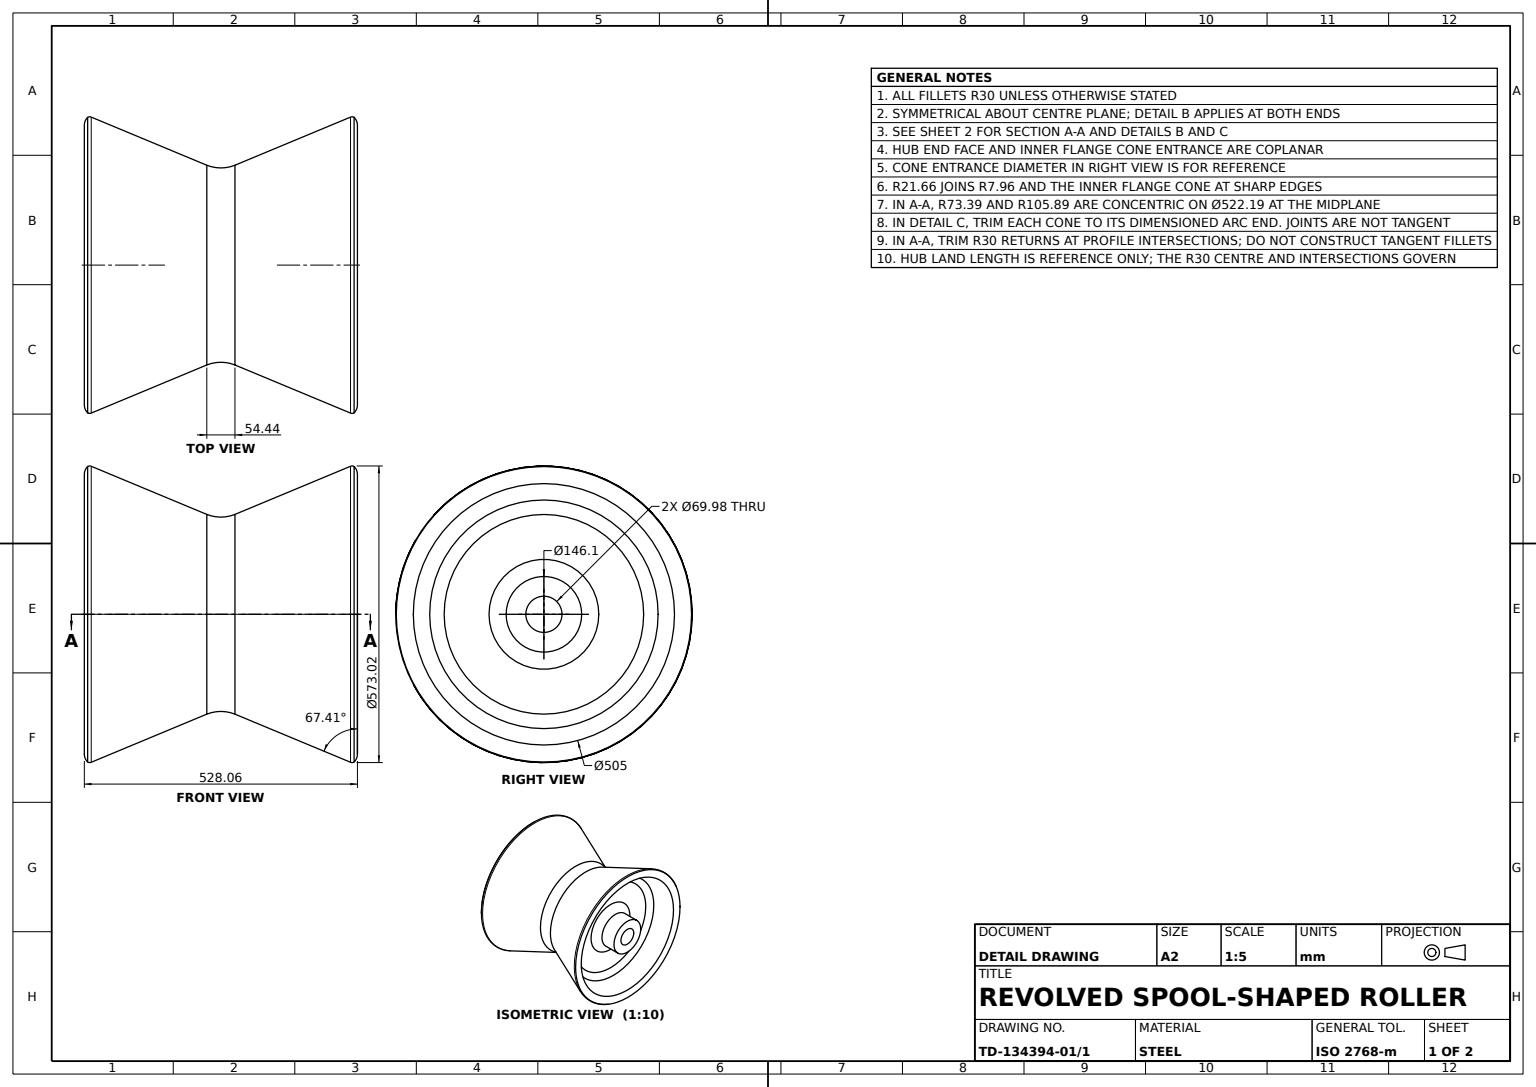
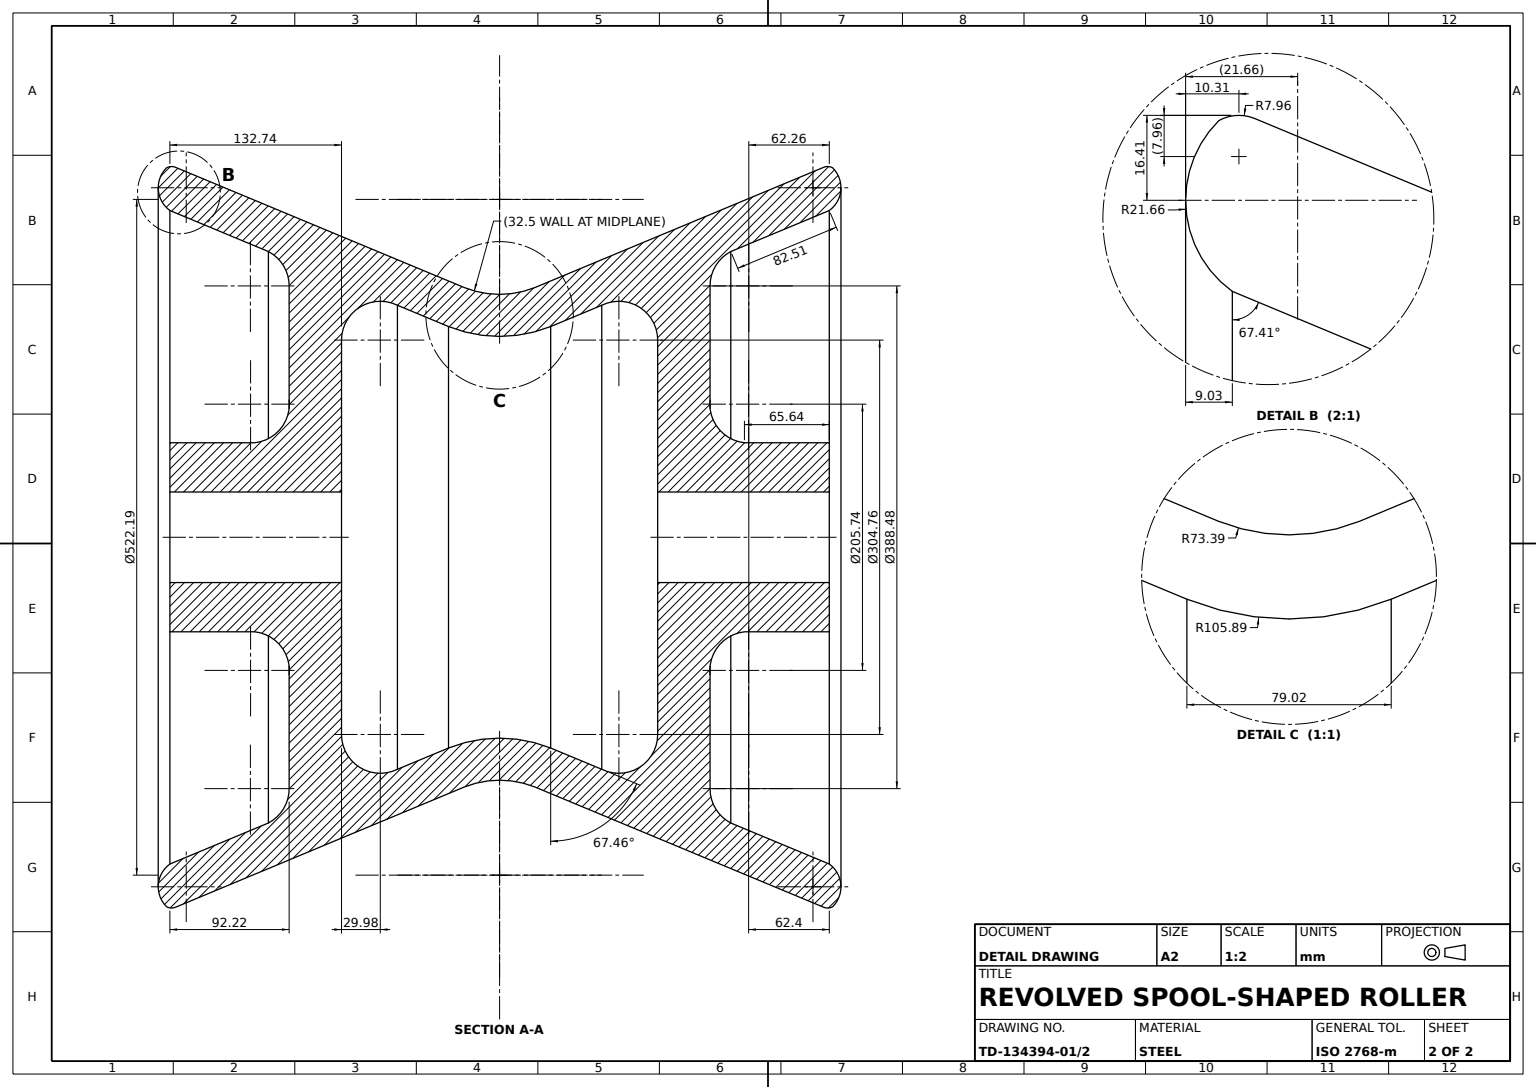
from build123d import *


with BuildPart() as part:
    # Cap Profile Sketch → Cap Body Revolve 360 (revolve)
    with BuildSketch(Plane.XY, mode=Mode.PRIVATE) as cap_body_revolve_360_sk:
        with BuildLine():
            Line((288.578542668, 183.908436408), (288.578542668, 67.489517857))
            Line((288.578542668, 67.489517857), (421.316369772, 67.489517857))
            Line((421.316369772, 67.489517857), (421.316369772, 105.548164289))
            Line((421.316369772, 105.548164289), (355.675042918, 105.548164289))
            ThreePointArc((355.675042918, 105.548164289), (335.535565441, 116.575822282), (329.092536094, 138.614315123))
            Line((329.092536094, 138.614315123), (329.092536094, 225.362437801))
            ThreePointArc((329.092536094, 225.362437801), (329.060998923, 226.737659861), (329.092536094, 228.112881921))
            ThreePointArc((329.092536094, 228.112881921), (333.753777304, 242.848045765), (345.131336453, 253.307652399))
            Line((345.131336453, 253.307652399), (421.316369772, 285.001353838))
            ThreePointArc((421.316369772, 285.001353838), (430.28137568, 300.893369363), (423.926034603, 317.997086158))
            ThreePointArc((423.926034603, 317.997086158), (420.516406834, 318.995196726), (417.01207704, 318.410851852))
            Line((417.01207704, 318.410851852), (236.369669575, 243.261885185))
            Line((236.369669575, 243.261885185), (193.537139087, 225.443143445))
            ThreePointArc((193.537139087, 225.443143445), (166.316369772, 220.208045956), (139.095600457, 225.443143445))
            Line((139.095600457, 225.443143445), (-84.379337496, 318.410851852))
            ThreePointArc((-84.379337496, 318.410851852), (-87.88366729, 318.995196726), (-91.29329506, 317.997086158))
            ThreePointArc((-91.29329506, 317.997086158), (-97.648636136, 300.893369363), (-88.683630228, 285.001353838))
            Line((-88.683630228, 285.001353838), (-12.498596909, 253.307652399))
            ThreePointArc((-12.498596909, 253.307652399), (-1.12103776, 242.848045765), (3.54020345, 228.112881921))
            ThreePointArc((3.54020345, 228.112881921), (3.571740621, 226.737659861), (3.54020345, 225.362437801))
            Line((3.54020345, 225.362437801), (3.54020345, 138.614315123))
            ThreePointArc((3.54020345, 138.614315123), (-2.902825897, 116.575822282), (-23.042303374, 105.548164289))
            Line((-23.042303374, 105.548164289), (-88.683630228, 105.548164289))
            Line((-88.683630228, 105.548164289), (-88.683630228, 67.489517857))
            Line((-88.683630228, 67.489517857), (44.054196876, 67.489517857))
            Line((44.054196876, 67.489517857), (44.054196876, 183.908436408))
            ThreePointArc((44.054196876, 183.908436408), (56.212998599, 209.010454978), (83.779873144, 213.254889383))
            ThreePointArc((83.779873144, 213.254889383), (85.561394381, 212.579290467), (87.296436491, 211.791965448))
            Line((87.296436491, 211.791965448), (126.806403131, 195.355441999))
            ThreePointArc((126.806403131, 195.355441999), (166.316369772, 187.708045956), (205.826336413, 195.355441999))
            Line((205.826336413, 195.355441999), (245.336303053, 211.791965448))
            ThreePointArc((245.336303053, 211.791965448), (247.071345163, 212.579290467), (248.8528664, 213.254889383))
            ThreePointArc((248.8528664, 213.254889383), (276.419740944, 209.010454978), (288.578542668, 183.908436408))
        make_face()
    revolve(cap_body_revolve_360_sk.sketch.rotate(Axis((-88.683630228, 32.5, 0), (1, 0, 0)), 90), axis=Axis((-88.683630228, 32.5, 0), (1, 0, 0)))


solid = part.part
